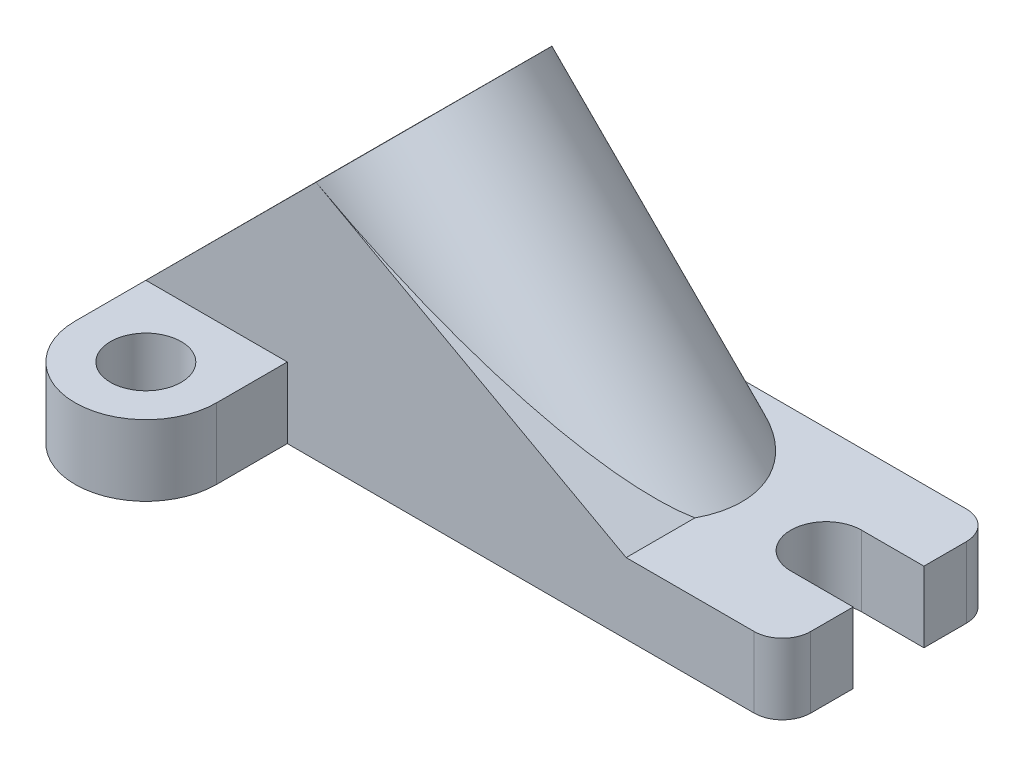
ISO-10303-21;
HEADER;
FILE_DESCRIPTION(('STEP AP214'),'2;1');
FILE_NAME('part.step','',(''),(''),'','','');
FILE_SCHEMA(('AUTOMOTIVE_DESIGN { 1 0 10303 214 1 1 1 1 }'));
ENDSEC;
DATA;
#1=APPLICATION_CONTEXT('core data for automotive mechanical design processes');
#2=APPLICATION_PROTOCOL_DEFINITION('international standard','automotive_design',2000,#1);
#3=PRODUCT_CONTEXT('',#1,'mechanical');
#4=PRODUCT('Part','Part','',(#3));
#5=PRODUCT_RELATED_PRODUCT_CATEGORY('part','',(#4));
#6=PRODUCT_DEFINITION_FORMATION('','',#4);
#7=PRODUCT_DEFINITION_CONTEXT('part definition',#1,'design');
#8=PRODUCT_DEFINITION('design','',#6,#7);
#9=PRODUCT_DEFINITION_SHAPE('','',#8);
#10=(LENGTH_UNIT() NAMED_UNIT(*) SI_UNIT(.MILLI.,.METRE.));
#11=(NAMED_UNIT(*) PLANE_ANGLE_UNIT() SI_UNIT($,.RADIAN.));
#12=(NAMED_UNIT(*) SI_UNIT($,.STERADIAN.) SOLID_ANGLE_UNIT());
#13=UNCERTAINTY_MEASURE_WITH_UNIT(LENGTH_MEASURE(1.E-05),#10,'distance_accuracy_value','');
#14=(GEOMETRIC_REPRESENTATION_CONTEXT(3) GLOBAL_UNCERTAINTY_ASSIGNED_CONTEXT((#13)) GLOBAL_UNIT_ASSIGNED_CONTEXT((#10,
#11,#12)) REPRESENTATION_CONTEXT('',''));
#15=CARTESIAN_POINT('',(0.,0.,0.));
#16=DIRECTION('',(0.,0.,1.));
#17=DIRECTION('',(1.,0.,0.));
#18=AXIS2_PLACEMENT_3D('',#15,#16,#17);
#19=CARTESIAN_POINT('',(24.0602572571438,29.0314215610274,-15.));
#20=DIRECTION('',(0.480628431220547,0.876924347422556,0.));
#21=DIRECTION('',(-0.876924347422556,0.480628431220547,0.));
#22=AXIS2_PLACEMENT_3D('',#19,#20,#21);
#23=PLANE('',#22);
#24=CARTESIAN_POINT('',(24.0602572571438,29.0314215610274,0.));
#25=DIRECTION('',(0.480628431220547,0.876924347422556,0.));
#26=DIRECTION('',(-0.876924347422556,0.480628431220547,0.));
#27=AXIS2_PLACEMENT_3D('',#24,#25,#26);
#28=ELLIPSE('',#27,53.4189832644045,15.);
#29=CARTESIAN_POINT('',(24.0602572571438,29.0314215610274,15.));
#30=VERTEX_POINT('',#29);
#31=CARTESIAN_POINT('',(67.9064746282716,5.,5.28012568938314));
#32=VERTEX_POINT('',#31);
#33=EDGE_CURVE('E11',#30,#32,#28,.T.);
#34=ORIENTED_EDGE('',*,*,#33,.F.);
#35=DIRECTION('',(-0.876924347422556,0.480628431220547,0.));
#36=VECTOR('',#35,1.);
#37=CARTESIAN_POINT('',(24.0602572571438,29.0314215610274,15.));
#38=LINE('',#37,#36);
#39=CARTESIAN_POINT('',(67.9064746282716,5.,15.));
#40=VERTEX_POINT('',#39);
#41=EDGE_CURVE('E207',#40,#30,#38,.T.);
#42=ORIENTED_EDGE('',*,*,#41,.F.);
#43=DIRECTION('',(0.,0.,1.));
#44=VECTOR('',#43,1.);
#45=CARTESIAN_POINT('',(67.9064746282716,5.,-15.));
#46=LINE('',#45,#44);
#47=EDGE_CURVE('E58',#32,#40,#46,.T.);
#48=ORIENTED_EDGE('',*,*,#47,.F.);
#49=EDGE_LOOP('',(#34,#42,#48));
#50=FACE_BOUND('',#49,.T.);
#51=ADVANCED_FACE('F41',(#50),#23,.T.);
#52=CARTESIAN_POINT('',(0.,5.,0.));
#53=DIRECTION('',(0.,1.,0.));
#54=DIRECTION('',(0.,0.,1.));
#55=AXIS2_PLACEMENT_3D('',#52,#53,#54);
#56=PLANE('',#55);
#57=CARTESIAN_POINT('',(10.,5.,-25.));
#58=DIRECTION('',(0.,1.,0.));
#59=DIRECTION('',(0.,0.,1.));
#60=AXIS2_PLACEMENT_3D('',#57,#58,#59);
#61=CIRCLE('',#60,5.);
#62=CARTESIAN_POINT('',(10.,5.,-20.));
#63=VERTEX_POINT('',#62);
#64=EDGE_CURVE('E257',#63,#63,#61,.T.);
#65=ORIENTED_EDGE('',*,*,#64,.F.);
#66=EDGE_LOOP('',(#65));
#67=FACE_BOUND('',#66,.T.);
#68=DIRECTION('',(0.,0.,-1.));
#69=VECTOR('',#68,1.);
#70=CARTESIAN_POINT('',(0.,5.,0.));
#71=LINE('',#70,#69);
#72=CARTESIAN_POINT('',(0.,5.,-15.));
#73=VERTEX_POINT('',#72);
#74=CARTESIAN_POINT('',(0.,5.,-25.));
#75=VERTEX_POINT('',#74);
#76=EDGE_CURVE('E239',#73,#75,#71,.T.);
#77=ORIENTED_EDGE('',*,*,#76,.F.);
#78=DIRECTION('',(1.,0.,0.));
#79=VECTOR('',#78,1.);
#80=CARTESIAN_POINT('',(0.,5.,-15.));
#81=LINE('',#80,#79);
#82=CARTESIAN_POINT('',(20.,5.,-15.));
#83=VERTEX_POINT('',#82);
#84=EDGE_CURVE('E201',#73,#83,#81,.T.);
#85=ORIENTED_EDGE('',*,*,#84,.T.);
#86=DIRECTION('',(0.,0.,1.));
#87=VECTOR('',#86,1.);
#88=CARTESIAN_POINT('',(20.,5.,0.));
#89=LINE('',#88,#87);
#90=CARTESIAN_POINT('',(20.,5.,-25.));
#91=VERTEX_POINT('',#90);
#92=EDGE_CURVE('E172',#91,#83,#89,.T.);
#93=ORIENTED_EDGE('',*,*,#92,.F.);
#94=CARTESIAN_POINT('',(10.,5.,-25.));
#95=DIRECTION('',(0.,1.,0.));
#96=DIRECTION('',(0.,0.,1.));
#97=AXIS2_PLACEMENT_3D('',#94,#95,#96);
#98=CIRCLE('',#97,10.);
#99=EDGE_CURVE('E240',#91,#75,#98,.T.);
#100=ORIENTED_EDGE('',*,*,#99,.T.);
#101=EDGE_LOOP('',(#77,#85,#93,#100));
#102=FACE_BOUND('',#101,.T.);
#103=ADVANCED_FACE('F393',(#67,#102),#56,.T.);
#104=CARTESIAN_POINT('',(48.0628776810106,5.,0.));
#105=DIRECTION('',(0.,1.,0.));
#106=DIRECTION('',(-1.,0.,0.));
#107=AXIS2_PLACEMENT_3D('',#104,#105,#106);
#108=ELLIPSE('',#107,21.2004954646264,15.);
#109=CARTESIAN_POINT('',(49.1800341683927,5.,-14.9791599353768));
#110=VERTEX_POINT('',#109);
#111=EDGE_CURVE('E57',#32,#110,#108,.T.);
#112=ORIENTED_EDGE('',*,*,#111,.F.);
#113=ORIENTED_EDGE('',*,*,#47,.T.);
#114=DIRECTION('',(-1.,0.,0.));
#115=VECTOR('',#114,1.);
#116=CARTESIAN_POINT('',(0.,5.,15.));
#117=LINE('',#116,#115);
#118=CARTESIAN_POINT('',(85.9999999999999,5.,15.));
#119=VERTEX_POINT('',#118);
#120=EDGE_CURVE('E249',#119,#40,#117,.T.);
#121=ORIENTED_EDGE('',*,*,#120,.F.);
#122=CARTESIAN_POINT('',(85.9999999999999,5.,11.));
#123=DIRECTION('',(0.,1.,0.));
#124=DIRECTION('',(0.,0.,1.));
#125=AXIS2_PLACEMENT_3D('',#122,#123,#124);
#126=CIRCLE('',#125,4.00000000000001);
#127=CARTESIAN_POINT('',(89.9999999999999,5.,11.));
#128=VERTEX_POINT('',#127);
#129=EDGE_CURVE('E213',#128,#119,#126,.F.);
#130=ORIENTED_EDGE('',*,*,#129,.F.);
#131=DIRECTION('',(0.,0.,1.));
#132=VECTOR('',#131,1.);
#133=CARTESIAN_POINT('',(90.,5.,8.32667268468869E-13));
#134=LINE('',#133,#132);
#135=CARTESIAN_POINT('',(90.,5.,5.));
#136=VERTEX_POINT('',#135);
#137=EDGE_CURVE('E216',#136,#128,#134,.T.);
#138=ORIENTED_EDGE('',*,*,#137,.F.);
#139=DIRECTION('',(1.,0.,0.));
#140=VECTOR('',#139,1.);
#141=CARTESIAN_POINT('',(0.,5.,4.99999999999999));
#142=LINE('',#141,#140);
#143=CARTESIAN_POINT('',(81.1772078264076,5.,5.));
#144=VERTEX_POINT('',#143);
#145=EDGE_CURVE('E225',#144,#136,#142,.T.);
#146=ORIENTED_EDGE('',*,*,#145,.F.);
#147=CARTESIAN_POINT('',(81.1772078264076,5.,0.));
#148=DIRECTION('',(0.,1.,0.));
#149=DIRECTION('',(0.,0.,1.));
#150=AXIS2_PLACEMENT_3D('',#147,#148,#149);
#151=CIRCLE('',#150,5.);
#152=CARTESIAN_POINT('',(81.1772078264076,5.,-5.));
#153=VERTEX_POINT('',#152);
#154=EDGE_CURVE('E224',#153,#144,#151,.T.);
#155=ORIENTED_EDGE('',*,*,#154,.F.);
#156=DIRECTION('',(-1.,0.,0.));
#157=VECTOR('',#156,1.);
#158=CARTESIAN_POINT('',(0.,5.,-4.99999999999999));
#159=LINE('',#158,#157);
#160=CARTESIAN_POINT('',(90.,5.,-5.));
#161=VERTEX_POINT('',#160);
#162=EDGE_CURVE('E226',#161,#153,#159,.T.);
#163=ORIENTED_EDGE('',*,*,#162,.F.);
#164=DIRECTION('',(0.,0.,1.));
#165=VECTOR('',#164,1.);
#166=CARTESIAN_POINT('',(90.,5.,0.));
#167=LINE('',#166,#165);
#168=CARTESIAN_POINT('',(90.,5.,-11.));
#169=VERTEX_POINT('',#168);
#170=EDGE_CURVE('E233',#169,#161,#167,.T.);
#171=ORIENTED_EDGE('',*,*,#170,.F.);
#172=CARTESIAN_POINT('',(86.,5.,-11.));
#173=DIRECTION('',(0.,1.,0.));
#174=DIRECTION('',(0.,0.,1.));
#175=AXIS2_PLACEMENT_3D('',#172,#173,#174);
#176=CIRCLE('',#175,4.00000000000001);
#177=CARTESIAN_POINT('',(86.,5.,-15.));
#178=VERTEX_POINT('',#177);
#179=EDGE_CURVE('E169',#169,#178,#176,.T.);
#180=ORIENTED_EDGE('',*,*,#179,.T.);
#181=DIRECTION('',(1.,0.,0.));
#182=VECTOR('',#181,1.);
#183=CARTESIAN_POINT('',(0.,5.,-15.));
#184=LINE('',#183,#182);
#185=CARTESIAN_POINT('',(49.1800341683927,5.,-15.));
#186=VERTEX_POINT('',#185);
#187=EDGE_CURVE('E161',#186,#178,#184,.T.);
#188=ORIENTED_EDGE('',*,*,#187,.F.);
#189=DIRECTION('',(0.,0.,-1.));
#190=VECTOR('',#189,1.);
#191=CARTESIAN_POINT('',(49.1800341683927,5.,60.3598880990025));
#192=LINE('',#191,#190);
#193=EDGE_CURVE('E168',#110,#186,#192,.T.);
#194=ORIENTED_EDGE('',*,*,#193,.F.);
#195=EDGE_LOOP('',(#112,#113,#121,#130,#138,#146,#155,#163,#171,#180,#188,#194));
#196=FACE_BOUND('',#195,.T.);
#197=ADVANCED_FACE('F164',(#196),#56,.T.);
#198=CARTESIAN_POINT('',(85.9999999999999,5.,11.));
#199=DIRECTION('',(0.,-1.,0.));
#200=DIRECTION('',(0.,0.,-1.));
#201=AXIS2_PLACEMENT_3D('',#198,#199,#200);
#202=CYLINDRICAL_SURFACE('',#201,4.00000000000001);
#203=CARTESIAN_POINT('',(85.9999999999999,-5.,11.));
#204=DIRECTION('',(0.,1.,0.));
#205=DIRECTION('',(0.,0.,1.));
#206=AXIS2_PLACEMENT_3D('',#203,#204,#205);
#207=CIRCLE('',#206,4.00000000000001);
#208=CARTESIAN_POINT('',(89.9999999999999,-5.,11.));
#209=VERTEX_POINT('',#208);
#210=CARTESIAN_POINT('',(85.9999999999999,-5.,15.));
#211=VERTEX_POINT('',#210);
#212=EDGE_CURVE('E214',#209,#211,#207,.F.);
#213=ORIENTED_EDGE('',*,*,#212,.F.);
#214=DIRECTION('',(0.,-1.,0.));
#215=VECTOR('',#214,1.);
#216=CARTESIAN_POINT('',(89.9999999999999,5.,11.));
#217=LINE('',#216,#215);
#218=EDGE_CURVE('E47',#128,#209,#217,.T.);
#219=ORIENTED_EDGE('',*,*,#218,.F.);
#220=ORIENTED_EDGE('',*,*,#129,.T.);
#221=DIRECTION('',(0.,-1.,0.));
#222=VECTOR('',#221,1.);
#223=CARTESIAN_POINT('',(85.9999999999999,5.,15.));
#224=LINE('',#223,#222);
#225=EDGE_CURVE('E256',#119,#211,#224,.T.);
#226=ORIENTED_EDGE('',*,*,#225,.T.);
#227=EDGE_LOOP('',(#213,#219,#220,#226));
#228=FACE_BOUND('',#227,.T.);
#229=ADVANCED_FACE('F43',(#228),#202,.T.);
#230=CARTESIAN_POINT('',(90.,5.,8.32667268468869E-13));
#231=DIRECTION('',(1.,0.,0.));
#232=DIRECTION('',(0.,0.,-1.));
#233=AXIS2_PLACEMENT_3D('',#230,#231,#232);
#234=PLANE('',#233);
#235=DIRECTION('',(0.,0.,1.));
#236=VECTOR('',#235,1.);
#237=CARTESIAN_POINT('',(90.,-5.,8.32667268468869E-13));
#238=LINE('',#237,#236);
#239=CARTESIAN_POINT('',(90.,-5.,5.));
#240=VERTEX_POINT('',#239);
#241=EDGE_CURVE('E265',#240,#209,#238,.T.);
#242=ORIENTED_EDGE('',*,*,#241,.F.);
#243=DIRECTION('',(0.,-1.,0.));
#244=VECTOR('',#243,1.);
#245=CARTESIAN_POINT('',(90.,5.,5.));
#246=LINE('',#245,#244);
#247=EDGE_CURVE('E326',#136,#240,#246,.T.);
#248=ORIENTED_EDGE('',*,*,#247,.F.);
#249=ORIENTED_EDGE('',*,*,#137,.T.);
#250=ORIENTED_EDGE('',*,*,#218,.T.);
#251=EDGE_LOOP('',(#242,#248,#249,#250));
#252=FACE_BOUND('',#251,.T.);
#253=ADVANCED_FACE('F335',(#252),#234,.T.);
#254=CARTESIAN_POINT('',(0.,5.,4.99999999999999));
#255=DIRECTION('',(0.,0.,-1.));
#256=DIRECTION('',(-1.,0.,0.));
#257=AXIS2_PLACEMENT_3D('',#254,#255,#256);
#258=PLANE('',#257);
#259=DIRECTION('',(1.,0.,0.));
#260=VECTOR('',#259,1.);
#261=CARTESIAN_POINT('',(0.,-5.,4.99999999999999));
#262=LINE('',#261,#260);
#263=CARTESIAN_POINT('',(81.1772078264076,-5.,5.));
#264=VERTEX_POINT('',#263);
#265=EDGE_CURVE('E262',#264,#240,#262,.T.);
#266=ORIENTED_EDGE('',*,*,#265,.F.);
#267=DIRECTION('',(0.,-1.,0.));
#268=VECTOR('',#267,1.);
#269=CARTESIAN_POINT('',(81.1772078264076,5.,5.));
#270=LINE('',#269,#268);
#271=EDGE_CURVE('E328',#144,#264,#270,.T.);
#272=ORIENTED_EDGE('',*,*,#271,.F.);
#273=ORIENTED_EDGE('',*,*,#145,.T.);
#274=ORIENTED_EDGE('',*,*,#247,.T.);
#275=EDGE_LOOP('',(#266,#272,#273,#274));
#276=FACE_BOUND('',#275,.T.);
#277=ADVANCED_FACE('F344',(#276),#258,.T.);
#278=CARTESIAN_POINT('',(81.1772078264076,5.,0.));
#279=DIRECTION('',(0.,-1.,0.));
#280=DIRECTION('',(0.,0.,-1.));
#281=AXIS2_PLACEMENT_3D('',#278,#279,#280);
#282=CYLINDRICAL_SURFACE('',#281,5.);
#283=CARTESIAN_POINT('',(81.1772078264076,-5.,0.));
#284=DIRECTION('',(0.,1.,0.));
#285=DIRECTION('',(0.,0.,1.));
#286=AXIS2_PLACEMENT_3D('',#283,#284,#285);
#287=CIRCLE('',#286,5.);
#288=CARTESIAN_POINT('',(81.1772078264076,-5.,-5.));
#289=VERTEX_POINT('',#288);
#290=EDGE_CURVE('E267',#289,#264,#287,.T.);
#291=ORIENTED_EDGE('',*,*,#290,.F.);
#292=DIRECTION('',(0.,-1.,0.));
#293=VECTOR('',#292,1.);
#294=CARTESIAN_POINT('',(81.1772078264076,5.,-5.));
#295=LINE('',#294,#293);
#296=EDGE_CURVE('E321',#153,#289,#295,.T.);
#297=ORIENTED_EDGE('',*,*,#296,.F.);
#298=ORIENTED_EDGE('',*,*,#154,.T.);
#299=ORIENTED_EDGE('',*,*,#271,.T.);
#300=EDGE_LOOP('',(#291,#297,#298,#299));
#301=FACE_BOUND('',#300,.T.);
#302=ADVANCED_FACE('F382',(#301),#282,.F.);
#303=CARTESIAN_POINT('',(0.,5.,-4.99999999999999));
#304=DIRECTION('',(0.,0.,1.));
#305=DIRECTION('',(1.,0.,0.));
#306=AXIS2_PLACEMENT_3D('',#303,#304,#305);
#307=PLANE('',#306);
#308=DIRECTION('',(-1.,0.,0.));
#309=VECTOR('',#308,1.);
#310=CARTESIAN_POINT('',(0.,-5.,-4.99999999999999));
#311=LINE('',#310,#309);
#312=CARTESIAN_POINT('',(90.,-5.,-5.));
#313=VERTEX_POINT('',#312);
#314=EDGE_CURVE('E272',#313,#289,#311,.T.);
#315=ORIENTED_EDGE('',*,*,#314,.F.);
#316=DIRECTION('',(0.,-1.,0.));
#317=VECTOR('',#316,1.);
#318=CARTESIAN_POINT('',(90.,5.,-5.));
#319=LINE('',#318,#317);
#320=EDGE_CURVE('E325',#161,#313,#319,.T.);
#321=ORIENTED_EDGE('',*,*,#320,.F.);
#322=ORIENTED_EDGE('',*,*,#162,.T.);
#323=ORIENTED_EDGE('',*,*,#296,.T.);
#324=EDGE_LOOP('',(#315,#321,#322,#323));
#325=FACE_BOUND('',#324,.T.);
#326=ADVANCED_FACE('F378',(#325),#307,.T.);
#327=CARTESIAN_POINT('',(90.,5.,0.));
#328=DIRECTION('',(1.,0.,0.));
#329=DIRECTION('',(0.,0.,-1.));
#330=AXIS2_PLACEMENT_3D('',#327,#328,#329);
#331=PLANE('',#330);
#332=DIRECTION('',(0.,0.,1.));
#333=VECTOR('',#332,1.);
#334=CARTESIAN_POINT('',(90.,-5.,0.));
#335=LINE('',#334,#333);
#336=CARTESIAN_POINT('',(90.,-5.,-11.));
#337=VERTEX_POINT('',#336);
#338=EDGE_CURVE('E274',#337,#313,#335,.T.);
#339=ORIENTED_EDGE('',*,*,#338,.F.);
#340=DIRECTION('',(0.,-1.,0.));
#341=VECTOR('',#340,1.);
#342=CARTESIAN_POINT('',(90.,5.,-11.));
#343=LINE('',#342,#341);
#344=EDGE_CURVE('E318',#169,#337,#343,.T.);
#345=ORIENTED_EDGE('',*,*,#344,.F.);
#346=ORIENTED_EDGE('',*,*,#170,.T.);
#347=ORIENTED_EDGE('',*,*,#320,.T.);
#348=EDGE_LOOP('',(#339,#345,#346,#347));
#349=FACE_BOUND('',#348,.T.);
#350=ADVANCED_FACE('F374',(#349),#331,.T.);
#351=CARTESIAN_POINT('',(86.,5.,-11.));
#352=DIRECTION('',(0.,-1.,0.));
#353=DIRECTION('',(0.,0.,-1.));
#354=AXIS2_PLACEMENT_3D('',#351,#352,#353);
#355=CYLINDRICAL_SURFACE('',#354,4.00000000000001);
#356=CARTESIAN_POINT('',(86.,-5.,-11.));
#357=DIRECTION('',(0.,1.,0.));
#358=DIRECTION('',(0.,0.,1.));
#359=AXIS2_PLACEMENT_3D('',#356,#357,#358);
#360=CIRCLE('',#359,4.00000000000001);
#361=CARTESIAN_POINT('',(86.,-5.,-15.));
#362=VERTEX_POINT('',#361);
#363=EDGE_CURVE('E280',#337,#362,#360,.T.);
#364=ORIENTED_EDGE('',*,*,#363,.T.);
#365=DIRECTION('',(0.,-1.,0.));
#366=VECTOR('',#365,1.);
#367=CARTESIAN_POINT('',(86.,5.,-15.));
#368=LINE('',#367,#366);
#369=EDGE_CURVE('E319',#178,#362,#368,.T.);
#370=ORIENTED_EDGE('',*,*,#369,.F.);
#371=ORIENTED_EDGE('',*,*,#179,.F.);
#372=ORIENTED_EDGE('',*,*,#344,.T.);
#373=EDGE_LOOP('',(#364,#370,#371,#372));
#374=FACE_BOUND('',#373,.T.);
#375=ADVANCED_FACE('F433',(#374),#355,.T.);
#376=CARTESIAN_POINT('',(0.,5.,-15.));
#377=DIRECTION('',(0.,0.,-1.));
#378=DIRECTION('',(-1.,0.,0.));
#379=AXIS2_PLACEMENT_3D('',#376,#377,#378);
#380=PLANE('',#379);
#381=DIRECTION('',(-0.722587126715869,0.691279859611507,0.));
#382=VECTOR('',#381,1.);
#383=CARTESIAN_POINT('',(49.1800341683927,5.,-15.));
#384=LINE('',#383,#382);
#385=CARTESIAN_POINT('',(24.0602572571438,29.0314215610274,-15.));
#386=VERTEX_POINT('',#385);
#387=EDGE_CURVE('E177',#186,#386,#384,.T.);
#388=ORIENTED_EDGE('',*,*,#387,.F.);
#389=ORIENTED_EDGE('',*,*,#187,.T.);
#390=ORIENTED_EDGE('',*,*,#369,.T.);
#391=DIRECTION('',(1.,0.,0.));
#392=VECTOR('',#391,1.);
#393=CARTESIAN_POINT('',(0.,-5.,-15.));
#394=LINE('',#393,#392);
#395=CARTESIAN_POINT('',(20.,-5.,-15.));
#396=VERTEX_POINT('',#395);
#397=EDGE_CURVE('E278',#396,#362,#394,.T.);
#398=ORIENTED_EDGE('',*,*,#397,.F.);
#399=DIRECTION('',(0.,-1.,0.));
#400=VECTOR('',#399,1.);
#401=CARTESIAN_POINT('',(20.,5.,-15.));
#402=LINE('',#401,#400);
#403=EDGE_CURVE('E317',#83,#396,#402,.T.);
#404=ORIENTED_EDGE('',*,*,#403,.F.);
#405=ORIENTED_EDGE('',*,*,#84,.F.);
#406=DIRECTION('',(-0.707530634132012,-0.706682674023322,0.));
#407=VECTOR('',#406,1.);
#408=CARTESIAN_POINT('',(0.,5.,-15.));
#409=LINE('',#408,#407);
#410=EDGE_CURVE('E187',#386,#73,#409,.T.);
#411=ORIENTED_EDGE('',*,*,#410,.F.);
#412=EDGE_LOOP('',(#388,#389,#390,#398,#404,#405,#411));
#413=FACE_BOUND('',#412,.T.);
#414=ADVANCED_FACE('F183',(#413),#380,.T.);
#415=CARTESIAN_POINT('',(20.,5.,0.));
#416=DIRECTION('',(1.,0.,0.));
#417=DIRECTION('',(0.,0.,-1.));
#418=AXIS2_PLACEMENT_3D('',#415,#416,#417);
#419=PLANE('',#418);
#420=DIRECTION('',(0.,0.,1.));
#421=VECTOR('',#420,1.);
#422=CARTESIAN_POINT('',(20.,-5.,0.));
#423=LINE('',#422,#421);
#424=CARTESIAN_POINT('',(20.,-5.,-25.));
#425=VERTEX_POINT('',#424);
#426=EDGE_CURVE('E285',#425,#396,#423,.T.);
#427=ORIENTED_EDGE('',*,*,#426,.F.);
#428=DIRECTION('',(0.,-1.,0.));
#429=VECTOR('',#428,1.);
#430=CARTESIAN_POINT('',(20.,5.,-25.));
#431=LINE('',#430,#429);
#432=EDGE_CURVE('E313',#91,#425,#431,.T.);
#433=ORIENTED_EDGE('',*,*,#432,.F.);
#434=ORIENTED_EDGE('',*,*,#92,.T.);
#435=ORIENTED_EDGE('',*,*,#403,.T.);
#436=EDGE_LOOP('',(#427,#433,#434,#435));
#437=FACE_BOUND('',#436,.T.);
#438=ADVANCED_FACE('F366',(#437),#419,.T.);
#439=CARTESIAN_POINT('',(10.,5.,-25.));
#440=DIRECTION('',(0.,-1.,0.));
#441=DIRECTION('',(0.,0.,-1.));
#442=AXIS2_PLACEMENT_3D('',#439,#440,#441);
#443=CYLINDRICAL_SURFACE('',#442,10.);
#444=CARTESIAN_POINT('',(10.,-5.,-25.));
#445=DIRECTION('',(0.,1.,0.));
#446=DIRECTION('',(0.,0.,1.));
#447=AXIS2_PLACEMENT_3D('',#444,#445,#446);
#448=CIRCLE('',#447,10.);
#449=CARTESIAN_POINT('',(0.,-5.,-25.));
#450=VERTEX_POINT('',#449);
#451=EDGE_CURVE('E282',#425,#450,#448,.T.);
#452=ORIENTED_EDGE('',*,*,#451,.T.);
#453=DIRECTION('',(0.,-1.,0.));
#454=VECTOR('',#453,1.);
#455=CARTESIAN_POINT('',(0.,5.,-25.));
#456=LINE('',#455,#454);
#457=EDGE_CURVE('E311',#75,#450,#456,.T.);
#458=ORIENTED_EDGE('',*,*,#457,.F.);
#459=ORIENTED_EDGE('',*,*,#99,.F.);
#460=ORIENTED_EDGE('',*,*,#432,.T.);
#461=EDGE_LOOP('',(#452,#458,#459,#460));
#462=FACE_BOUND('',#461,.T.);
#463=ADVANCED_FACE('F428',(#462),#443,.T.);
#464=CARTESIAN_POINT('',(0.,5.,0.));
#465=DIRECTION('',(-1.,0.,0.));
#466=DIRECTION('',(0.,0.,1.));
#467=AXIS2_PLACEMENT_3D('',#464,#465,#466);
#468=PLANE('',#467);
#469=DIRECTION('',(0.,0.,-1.));
#470=VECTOR('',#469,1.);
#471=CARTESIAN_POINT('',(0.,-5.,0.));
#472=LINE('',#471,#470);
#473=CARTESIAN_POINT('',(0.,-5.,25.));
#474=VERTEX_POINT('',#473);
#475=EDGE_CURVE('E287',#474,#450,#472,.T.);
#476=ORIENTED_EDGE('',*,*,#475,.F.);
#477=DIRECTION('',(0.,-1.,0.));
#478=VECTOR('',#477,1.);
#479=CARTESIAN_POINT('',(0.,5.,25.));
#480=LINE('',#479,#478);
#481=CARTESIAN_POINT('',(0.,5.,25.));
#482=VERTEX_POINT('',#481);
#483=EDGE_CURVE('E307',#482,#474,#480,.T.);
#484=ORIENTED_EDGE('',*,*,#483,.F.);
#485=CARTESIAN_POINT('',(0.,5.,15.));
#486=VERTEX_POINT('',#485);
#487=EDGE_CURVE('E241',#482,#486,#71,.T.);
#488=ORIENTED_EDGE('',*,*,#487,.T.);
#489=DIRECTION('',(0.,0.,1.));
#490=VECTOR('',#489,1.);
#491=CARTESIAN_POINT('',(0.,5.,-15.));
#492=LINE('',#491,#490);
#493=EDGE_CURVE('E212',#73,#486,#492,.T.);
#494=ORIENTED_EDGE('',*,*,#493,.F.);
#495=ORIENTED_EDGE('',*,*,#76,.T.);
#496=ORIENTED_EDGE('',*,*,#457,.T.);
#497=EDGE_LOOP('',(#476,#484,#488,#494,#495,#496));
#498=FACE_BOUND('',#497,.T.);
#499=ADVANCED_FACE('F359',(#498),#468,.T.);
#500=CARTESIAN_POINT('',(9.99999999999999,5.,25.));
#501=DIRECTION('',(0.,-1.,0.));
#502=DIRECTION('',(0.,0.,-1.));
#503=AXIS2_PLACEMENT_3D('',#500,#501,#502);
#504=CYLINDRICAL_SURFACE('',#503,9.99999999999999);
#505=CARTESIAN_POINT('',(9.99999999999999,-5.,25.));
#506=DIRECTION('',(0.,1.,0.));
#507=DIRECTION('',(0.,0.,1.));
#508=AXIS2_PLACEMENT_3D('',#505,#506,#507);
#509=CIRCLE('',#508,9.99999999999999);
#510=CARTESIAN_POINT('',(20.,-5.,25.));
#511=VERTEX_POINT('',#510);
#512=EDGE_CURVE('E289',#511,#474,#509,.F.);
#513=ORIENTED_EDGE('',*,*,#512,.F.);
#514=DIRECTION('',(0.,-1.,0.));
#515=VECTOR('',#514,1.);
#516=CARTESIAN_POINT('',(20.,5.,25.));
#517=LINE('',#516,#515);
#518=CARTESIAN_POINT('',(20.,5.,25.));
#519=VERTEX_POINT('',#518);
#520=EDGE_CURVE('E310',#519,#511,#517,.T.);
#521=ORIENTED_EDGE('',*,*,#520,.F.);
#522=CARTESIAN_POINT('',(9.99999999999999,5.,25.));
#523=DIRECTION('',(0.,1.,0.));
#524=DIRECTION('',(0.,0.,1.));
#525=AXIS2_PLACEMENT_3D('',#522,#523,#524);
#526=CIRCLE('',#525,9.99999999999999);
#527=EDGE_CURVE('E242',#519,#482,#526,.F.);
#528=ORIENTED_EDGE('',*,*,#527,.T.);
#529=ORIENTED_EDGE('',*,*,#483,.T.);
#530=EDGE_LOOP('',(#513,#521,#528,#529));
#531=FACE_BOUND('',#530,.T.);
#532=ADVANCED_FACE('F353',(#531),#504,.T.);
#533=CARTESIAN_POINT('',(20.,5.,0.));
#534=DIRECTION('',(-1.,0.,0.));
#535=DIRECTION('',(0.,0.,1.));
#536=AXIS2_PLACEMENT_3D('',#533,#534,#535);
#537=PLANE('',#536);
#538=DIRECTION('',(0.,0.,-1.));
#539=VECTOR('',#538,1.);
#540=CARTESIAN_POINT('',(20.,-5.,0.));
#541=LINE('',#540,#539);
#542=CARTESIAN_POINT('',(20.,-5.,15.));
#543=VERTEX_POINT('',#542);
#544=EDGE_CURVE('E291',#511,#543,#541,.T.);
#545=ORIENTED_EDGE('',*,*,#544,.T.);
#546=DIRECTION('',(0.,-1.,0.));
#547=VECTOR('',#546,1.);
#548=CARTESIAN_POINT('',(20.,5.,15.));
#549=LINE('',#548,#547);
#550=CARTESIAN_POINT('',(20.,5.,15.));
#551=VERTEX_POINT('',#550);
#552=EDGE_CURVE('E302',#551,#543,#549,.T.);
#553=ORIENTED_EDGE('',*,*,#552,.F.);
#554=DIRECTION('',(0.,0.,-1.));
#555=VECTOR('',#554,1.);
#556=CARTESIAN_POINT('',(20.,5.,0.));
#557=LINE('',#556,#555);
#558=EDGE_CURVE('E250',#519,#551,#557,.T.);
#559=ORIENTED_EDGE('',*,*,#558,.F.);
#560=ORIENTED_EDGE('',*,*,#520,.T.);
#561=EDGE_LOOP('',(#545,#553,#559,#560));
#562=FACE_BOUND('',#561,.T.);
#563=ADVANCED_FACE('F420',(#562),#537,.F.);
#564=CARTESIAN_POINT('',(9.99999999999999,5.,25.));
#565=DIRECTION('',(0.,-1.,0.));
#566=DIRECTION('',(0.,0.,-1.));
#567=AXIS2_PLACEMENT_3D('',#564,#565,#566);
#568=CYLINDRICAL_SURFACE('',#567,5.);
#569=CARTESIAN_POINT('',(9.99999999999999,5.,25.));
#570=DIRECTION('',(0.,1.,0.));
#571=DIRECTION('',(0.,0.,1.));
#572=AXIS2_PLACEMENT_3D('',#569,#570,#571);
#573=CIRCLE('',#572,5.);
#574=CARTESIAN_POINT('',(9.99999999999999,5.,30.));
#575=VERTEX_POINT('',#574);
#576=EDGE_CURVE('E254',#575,#575,#573,.F.);
#577=ORIENTED_EDGE('',*,*,#576,.F.);
#578=EDGE_LOOP('',(#577));
#579=FACE_BOUND('',#578,.T.);
#580=CARTESIAN_POINT('',(9.99999999999999,-5.,25.));
#581=DIRECTION('',(0.,1.,0.));
#582=DIRECTION('',(0.,0.,1.));
#583=AXIS2_PLACEMENT_3D('',#580,#581,#582);
#584=CIRCLE('',#583,5.);
#585=CARTESIAN_POINT('',(9.99999999999999,-5.,30.));
#586=VERTEX_POINT('',#585);
#587=EDGE_CURVE('E296',#586,#586,#584,.F.);
#588=ORIENTED_EDGE('',*,*,#587,.T.);
#589=EDGE_LOOP('',(#588));
#590=FACE_BOUND('',#589,.T.);
#591=ADVANCED_FACE('F414',(#579,#590),#568,.F.);
#592=CARTESIAN_POINT('',(0.,5.,15.));
#593=DIRECTION('',(0.,0.,1.));
#594=DIRECTION('',(1.,0.,0.));
#595=AXIS2_PLACEMENT_3D('',#592,#593,#594);
#596=PLANE('',#595);
#597=ORIENTED_EDGE('',*,*,#41,.T.);
#598=DIRECTION('',(-0.707530634132012,-0.706682674023322,0.));
#599=VECTOR('',#598,1.);
#600=CARTESIAN_POINT('',(0.,5.,15.));
#601=LINE('',#600,#599);
#602=EDGE_CURVE('E202',#30,#486,#601,.T.);
#603=ORIENTED_EDGE('',*,*,#602,.T.);
#604=DIRECTION('',(1.,0.,0.));
#605=VECTOR('',#604,1.);
#606=CARTESIAN_POINT('',(0.,5.,15.));
#607=LINE('',#606,#605);
#608=EDGE_CURVE('E197',#486,#551,#607,.T.);
#609=ORIENTED_EDGE('',*,*,#608,.T.);
#610=ORIENTED_EDGE('',*,*,#552,.T.);
#611=DIRECTION('',(-1.,0.,0.));
#612=VECTOR('',#611,1.);
#613=CARTESIAN_POINT('',(0.,-5.,15.));
#614=LINE('',#613,#612);
#615=EDGE_CURVE('E298',#211,#543,#614,.T.);
#616=ORIENTED_EDGE('',*,*,#615,.F.);
#617=ORIENTED_EDGE('',*,*,#225,.F.);
#618=ORIENTED_EDGE('',*,*,#120,.T.);
#619=EDGE_LOOP('',(#597,#603,#609,#610,#616,#617,#618));
#620=FACE_BOUND('',#619,.T.);
#621=ADVANCED_FACE('F350',(#620),#596,.T.);
#622=CARTESIAN_POINT('',(10.,5.,-25.));
#623=DIRECTION('',(0.,-1.,0.));
#624=DIRECTION('',(0.,0.,-1.));
#625=AXIS2_PLACEMENT_3D('',#622,#623,#624);
#626=CYLINDRICAL_SURFACE('',#625,5.);
#627=ORIENTED_EDGE('',*,*,#64,.T.);
#628=EDGE_LOOP('',(#627));
#629=FACE_BOUND('',#628,.T.);
#630=CARTESIAN_POINT('',(10.,-5.,-25.));
#631=DIRECTION('',(0.,1.,0.));
#632=DIRECTION('',(0.,0.,1.));
#633=AXIS2_PLACEMENT_3D('',#630,#631,#632);
#634=CIRCLE('',#633,5.);
#635=CARTESIAN_POINT('',(10.,-5.,-20.));
#636=VERTEX_POINT('',#635);
#637=EDGE_CURVE('E219',#636,#636,#634,.T.);
#638=ORIENTED_EDGE('',*,*,#637,.F.);
#639=EDGE_LOOP('',(#638));
#640=FACE_BOUND('',#639,.T.);
#641=ADVANCED_FACE('F407',(#629,#640),#626,.F.);
#642=ORIENTED_EDGE('',*,*,#608,.F.);
#643=ORIENTED_EDGE('',*,*,#487,.F.);
#644=ORIENTED_EDGE('',*,*,#527,.F.);
#645=ORIENTED_EDGE('',*,*,#558,.T.);
#646=EDGE_LOOP('',(#642,#643,#644,#645));
#647=FACE_BOUND('',#646,.T.);
#648=ORIENTED_EDGE('',*,*,#576,.T.);
#649=EDGE_LOOP('',(#648));
#650=FACE_BOUND('',#649,.T.);
#651=ADVANCED_FACE('F402',(#647,#650),#56,.T.);
#652=CARTESIAN_POINT('',(0.,-5.,0.));
#653=DIRECTION('',(0.,1.,0.));
#654=DIRECTION('',(0.,0.,1.));
#655=AXIS2_PLACEMENT_3D('',#652,#653,#654);
#656=PLANE('',#655);
#657=CARTESIAN_POINT('',(58.0508928980516,-5.,0.));
#658=DIRECTION('',(0.,1.,0.));
#659=DIRECTION('',(-1.,0.,0.));
#660=AXIS2_PLACEMENT_3D('',#657,#658,#659);
#661=ELLIPSE('',#660,10.6002477323132,7.5);
#662=CARTESIAN_POINT('',(47.4506451657384,-5.,0.));
#663=VERTEX_POINT('',#662);
#664=EDGE_CURVE('E191',#663,#663,#661,.T.);
#665=ORIENTED_EDGE('',*,*,#664,.T.);
#666=EDGE_LOOP('',(#665));
#667=FACE_BOUND('',#666,.T.);
#668=ORIENTED_EDGE('',*,*,#615,.T.);
#669=ORIENTED_EDGE('',*,*,#544,.F.);
#670=ORIENTED_EDGE('',*,*,#512,.T.);
#671=ORIENTED_EDGE('',*,*,#475,.T.);
#672=ORIENTED_EDGE('',*,*,#451,.F.);
#673=ORIENTED_EDGE('',*,*,#426,.T.);
#674=ORIENTED_EDGE('',*,*,#397,.T.);
#675=ORIENTED_EDGE('',*,*,#363,.F.);
#676=ORIENTED_EDGE('',*,*,#338,.T.);
#677=ORIENTED_EDGE('',*,*,#314,.T.);
#678=ORIENTED_EDGE('',*,*,#290,.T.);
#679=ORIENTED_EDGE('',*,*,#265,.T.);
#680=ORIENTED_EDGE('',*,*,#241,.T.);
#681=ORIENTED_EDGE('',*,*,#212,.T.);
#682=EDGE_LOOP('',(#668,#669,#670,#671,#672,#673,#674,#675,#676,#677,#678,#679,#680,#681));
#683=FACE_BOUND('',#682,.T.);
#684=ORIENTED_EDGE('',*,*,#587,.F.);
#685=EDGE_LOOP('',(#684));
#686=FACE_BOUND('',#685,.T.);
#687=ORIENTED_EDGE('',*,*,#637,.T.);
#688=EDGE_LOOP('',(#687));
#689=FACE_BOUND('',#688,.T.);
#690=ADVANCED_FACE('F336',(#667,#683,#686,#689),#656,.F.);
#691=CARTESIAN_POINT('',(0.,5.,-15.));
#692=DIRECTION('',(-0.706682674023322,0.707530634132012,0.));
#693=DIRECTION('',(-0.707530634132012,-0.706682674023322,0.));
#694=AXIS2_PLACEMENT_3D('',#691,#692,#693);
#695=PLANE('',#694);
#696=CARTESIAN_POINT('',(24.0602572571438,29.0314215610273,0.));
#697=DIRECTION('',(-0.706682674023322,0.707530634132013,0.));
#698=DIRECTION('',(-0.707530634132013,-0.706682674023322,0.));
#699=AXIS2_PLACEMENT_3D('',#696,#697,#698);
#700=CIRCLE('',#699,7.5);
#701=CARTESIAN_POINT('',(18.7537775011537,23.7313015058524,0.));
#702=VERTEX_POINT('',#701);
#703=EDGE_CURVE('E192',#702,#702,#700,.T.);
#704=ORIENTED_EDGE('',*,*,#703,.F.);
#705=EDGE_LOOP('',(#704));
#706=FACE_BOUND('',#705,.T.);
#707=ORIENTED_EDGE('',*,*,#602,.F.);
#708=CARTESIAN_POINT('',(24.0602572571438,29.0314215610273,0.));
#709=DIRECTION('',(-0.706682674023322,0.707530634132013,0.));
#710=DIRECTION('',(-0.707530634132013,-0.706682674023322,0.));
#711=AXIS2_PLACEMENT_3D('',#708,#709,#710);
#712=CIRCLE('',#711,15.);
#713=EDGE_CURVE('E200',#30,#386,#712,.T.);
#714=ORIENTED_EDGE('',*,*,#713,.T.);
#715=ORIENTED_EDGE('',*,*,#410,.T.);
#716=ORIENTED_EDGE('',*,*,#493,.T.);
#717=EDGE_LOOP('',(#707,#714,#715,#716));
#718=FACE_BOUND('',#717,.T.);
#719=ADVANCED_FACE('F401',(#706,#718),#695,.T.);
#720=CARTESIAN_POINT('',(62.9278043284265,-9.88276331623335,0.));
#721=DIRECTION('',(-0.706682674023322,0.707530634132013,0.));
#722=DIRECTION('',(-0.707530634132013,-0.706682674023322,0.));
#723=AXIS2_PLACEMENT_3D('',#720,#721,#722);
#724=CYLINDRICAL_SURFACE('',#723,15.);
#725=ORIENTED_EDGE('',*,*,#713,.F.);
#726=ORIENTED_EDGE('',*,*,#33,.T.);
#727=ORIENTED_EDGE('',*,*,#111,.T.);
#728=CARTESIAN_POINT('',(24.0602572571436,29.0314215610276,0.));
#729=DIRECTION('',(-0.691279859611507,-0.722587126715869,0.));
#730=DIRECTION('',(-0.722587126715869,0.691279859611507,0.));
#731=AXIS2_PLACEMENT_3D('',#728,#729,#730);
#732=ELLIPSE('',#731,659.716819948625,15.);
#733=EDGE_CURVE('E181',#386,#110,#732,.T.);
#734=ORIENTED_EDGE('',*,*,#733,.F.);
#735=EDGE_LOOP('',(#725,#726,#727,#734));
#736=FACE_BOUND('',#735,.T.);
#737=ADVANCED_FACE('F555',(#736),#724,.T.);
#738=CARTESIAN_POINT('',(66.4612176985431,-13.4204164868934,0.));
#739=DIRECTION('',(-0.706682674023322,0.707530634132013,0.));
#740=DIRECTION('',(-0.707530634132013,-0.706682674023322,0.));
#741=AXIS2_PLACEMENT_3D('',#738,#739,#740);
#742=CYLINDRICAL_SURFACE('',#741,7.5);
#743=ORIENTED_EDGE('',*,*,#703,.T.);
#744=EDGE_LOOP('',(#743));
#745=FACE_BOUND('',#744,.T.);
#746=ORIENTED_EDGE('',*,*,#664,.F.);
#747=EDGE_LOOP('',(#746));
#748=FACE_BOUND('',#747,.T.);
#749=ADVANCED_FACE('F566',(#745,#748),#742,.F.);
#750=CARTESIAN_POINT('',(49.1800341683927,5.,60.3598880990025));
#751=DIRECTION('',(-0.691279859611507,-0.722587126715869,0.));
#752=DIRECTION('',(0.722587126715869,-0.691279859611507,0.));
#753=AXIS2_PLACEMENT_3D('',#750,#751,#752);
#754=PLANE('',#753);
#755=ORIENTED_EDGE('',*,*,#733,.T.);
#756=ORIENTED_EDGE('',*,*,#193,.T.);
#757=ORIENTED_EDGE('',*,*,#387,.T.);
#758=EDGE_LOOP('',(#755,#756,#757));
#759=FACE_BOUND('',#758,.T.);
#760=ADVANCED_FACE('F178',(#759),#754,.F.);
#761=CLOSED_SHELL('',(#51,#103,#197,#229,#253,#277,#302,#326,#350,#375,#414,#438,#463,#499,#532,
#563,#591,#621,#641,#651,#690,#719,#737,#749,#760));
#762=MANIFOLD_SOLID_BREP('B2',#761);
#763=ADVANCED_BREP_SHAPE_REPRESENTATION('',(#18,#762),#14);
#764=SHAPE_DEFINITION_REPRESENTATION(#9,#763);
ENDSEC;
END-ISO-10303-21;
